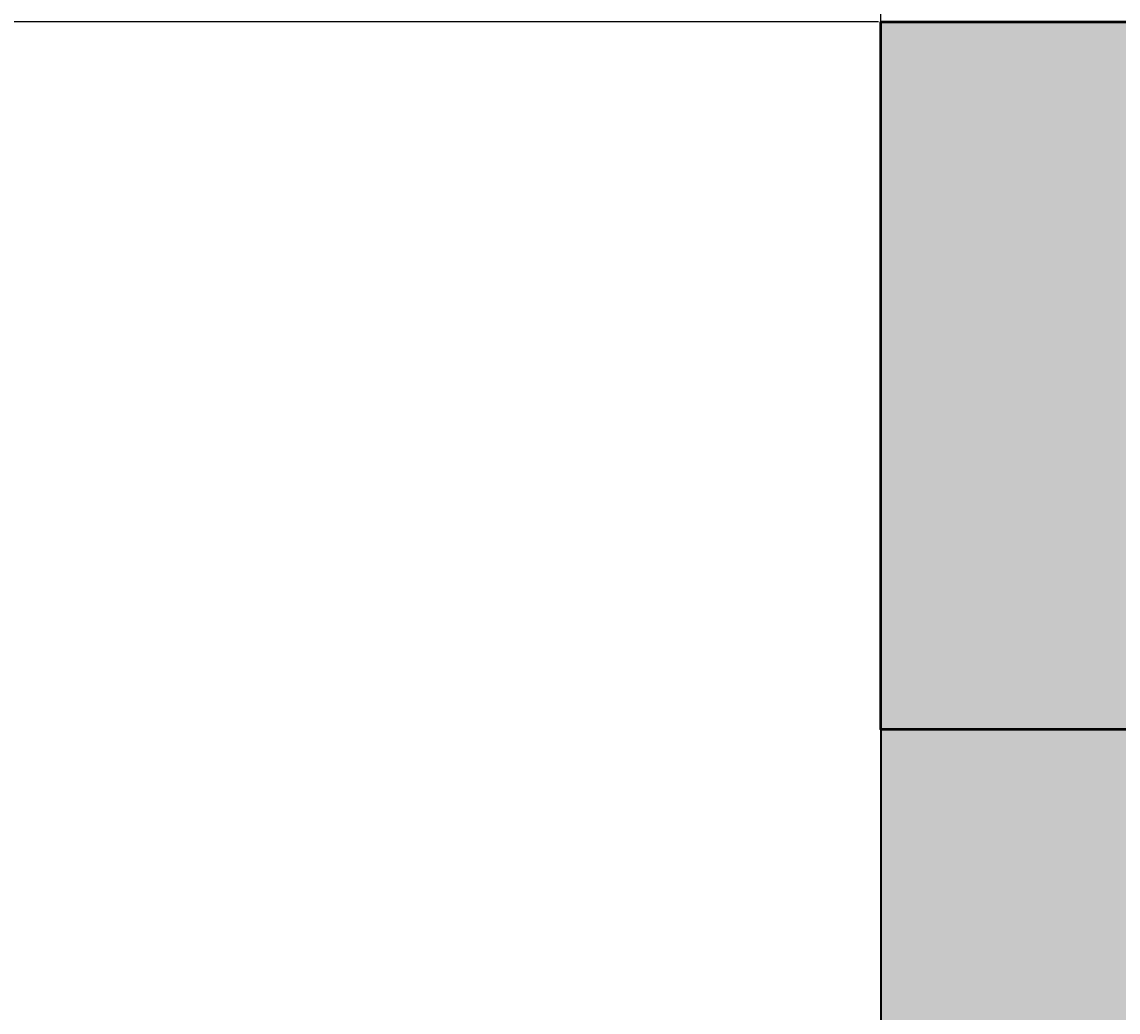
# Model space of a CAD drawing. Units: inches. Extents: x 1998 to 2588, y 1139 to 1977.
# Tile 71 of 134: x 2063 to 2095, y 1860 to 1889. Entities that reach past the tile are written whole.
import ezdxf

# ---------------------------------------------------------------- set-up
doc = ezdxf.new("R2010")
doc.units = ezdxf.units.IN
for name, color, linetype, lineweight in [('A-ANNO-DIMS', 2, 'Continuous', 18), ('A-COLS-PATT', 250, 'Continuous', 13), ('A-WALL-PATT', 252, 'Continuous', 13), ('COLUMN', 10, 'Continuous', 50), ('WALL', 200, 'Continuous', 35)]:
    doc.layers.add(name, color=color, linetype=linetype, lineweight=lineweight)
doc.styles.get("Standard").update_dxf_attribs({"font": 'arial.ttf'})
doc.dimstyles.get("Standard").update_dxf_attribs({"dimtxt": 0.18, "dimasz": 0.18, "dimexe": 0.18, "dimexo": 0.0625, "dimgap": 0.09, "dimtad": 0, "dimtih": 1, "dimtoh": 1, "dimdec": 4, "dimzin": 0, "dimdsep": 46, "dimtxsty": 'Standard', "dimcen": 0.09, "dimadec": 0, "dimazin": 0, "dimtfac": 1, "dimtdec": 4, "dimtofl": 0, "dimtmove": 0, "dimatfit": 3, "dimfxl": 1, "dimtolj": 1, "dimtzin": 0, "dimarcsym": 0})

# ---------------------------------------------------------------- blocks, each defined once
blk = doc.blocks.new('*D28')
at = {"layer": 'A-ANNO-DIMS', "color": 0, "lineweight": -2, "transparency": 16777216}
for p, q in [((2059.473, 1759.795), (2059.473, 1977.362)), ((2087.973, 1759.795), (2087.973, 1977.362)), ((2059.653, 1977.182), (2073.397, 1977.182)), ((2087.793, 1977.182), (2074.049, 1977.182))]:
    blk.add_line(p, q, dxfattribs=at)
at = {"layer": 'A-ANNO-DIMS', "color": 0, "transparency": 16777216}
for points in [[(2059.653, 1977.212), (2059.653, 1977.152), (2059.473, 1977.182)], [(2087.793, 1977.212), (2087.793, 1977.152), (2087.973, 1977.182)]]:
    blk.add_solid(points, dxfattribs=at)
at = {"layer": 'Defpoints', "color": 0, "transparency": 16777216}
for p in [(2087.973, 1977.182), (2059.473, 1759.732), (2087.973, 1759.732)]:
    blk.add_point(p, dxfattribs=at)
at = {"layer": 'A-ANNO-DIMS', "color": 0, "transparency": 16777216, "insert": (2073.723, 1977.182), "char_height": 0.18, "attachment_point": 5}
blk.add_mtext('\\A1;28.5', dxfattribs=at)
blk = doc.blocks.new('*D29')
at = {"layer": 'A-ANNO-DIMS', "color": 0, "lineweight": -2, "transparency": 16777216}
for p, q in [((2087.91, 1888.732), (1997.843, 1888.732)), ((1998.023, 1888.552), (1998.023, 1824.414)), ((1998.023, 1759.912), (1998.023, 1824.05)), ((2059.41, 1759.732), (1997.843, 1759.732))]:
    blk.add_line(p, q, dxfattribs=at)
at = {"layer": 'A-ANNO-DIMS', "color": 0, "transparency": 16777216}
for points in [[(1997.993, 1888.552), (1998.053, 1888.552), (1998.023, 1888.732)], [(1997.993, 1759.912), (1998.053, 1759.912), (1998.023, 1759.732)]]:
    blk.add_solid(points, dxfattribs=at)
at = {"layer": 'Defpoints', "color": 0, "transparency": 16777216}
for p in [(1998.023, 1888.732), (2087.973, 1888.732), (2059.473, 1759.732)]:
    blk.add_point(p, dxfattribs=at)
at = {"layer": 'A-ANNO-DIMS', "color": 0, "transparency": 16777216, "insert": (1998.023, 1824.232), "char_height": 0.18, "attachment_point": 5}
blk.add_mtext('\\A1;129', dxfattribs=at)

msp = doc.modelspace()

# ---------------------------------------------------------------- hatches: boundary and pattern name
at = {"layer": 'A-COLS-PATT'}
h = msp.add_hatch(color=256, dxfattribs=at)
h.dxf.hatch_style = 1
h.paths.add_polyline_path([(2099.4125, 1888.7324), (2087.9729, 1888.7324), (2087.9729, 1868.3278), (2099.4125, 1868.3278)])
h.paths.add_polyline_path([(2234.4125, 1888.7324), (2222.9729, 1888.7324), (2222.9729, 1868.3278), (2234.4125, 1868.3278)])
h.paths.add_polyline_path([(2341.4729, 1886.637), (2330.0332, 1886.637), (2330.0332, 1866.2324), (2341.4729, 1866.2324)])
h.paths.add_polyline_path([(2507.8006, 1882.7324), (2487.396, 1882.7324), (2487.396, 1871.2927), (2507.8006, 1871.2927)])
h.paths.add_polyline_path([(2510.9729, 1766.672), (2490.5682, 1766.672), (2490.5682, 1755.2324), (2510.9729, 1755.2324)])
h.paths.add_polyline_path([(2345.9729, 1759.7324), (2334.5332, 1759.7324), (2334.5332, 1739.3278), (2345.9729, 1739.3278)])
h.paths.add_polyline_path([(2234.4125, 1774.3318), (2222.9729, 1774.3318), (2222.9729, 1753.9272), (2234.4125, 1753.9272)])
h.paths.add_polyline_path([(2099.4125, 1775.637), (2087.9729, 1775.637), (2087.9729, 1755.2324), (2099.4125, 1755.2324)])
h.paths.add_polyline_path([(2098.0956, 1593.7241), (2077.691, 1593.7241), (2077.691, 1582.2845), (2098.0956, 1582.2845)])
h.paths.add_polyline_path([(2227.4729, 1604.637), (2216.0332, 1604.637), (2216.0332, 1584.2324), (2227.4729, 1584.2324)])
h.paths.add_polyline_path([(2345.9729, 1647.5211), (2334.5332, 1647.5211), (2334.5332, 1627.1165), (2345.9729, 1627.1165)])
h.paths.add_polyline_path([(2522.3775, 1641.2324), (2501.9729, 1641.2324), (2501.9729, 1629.7927), (2522.3775, 1629.7927)])
h.paths.add_polyline_path([(2522.3775, 1480.7324), (2501.9729, 1480.7324), (2501.9729, 1469.2927), (2522.3775, 1469.2927)])
h.paths.add_polyline_path([(2345.9729, 1488.5616), (2334.5332, 1488.5616), (2334.5332, 1468.1569), (2345.9729, 1468.1569)])
h.paths.add_polyline_path([(2234.4125, 1486.137), (2227.4729, 1486.137), (2227.4729, 1465.7324), (2234.4125, 1465.7324)])
h.paths.add_polyline_path([(2227.4729, 1486.137), (2222.9729, 1486.137), (2222.9729, 1465.7324), (2227.4729, 1465.7324)])
h.paths.add_polyline_path([(2108.3775, 1470.2324), (2087.9729, 1470.2324), (2087.9729, 1458.7927), (2108.3775, 1458.7927)])
h.paths.add_polyline_path([(2096.9729, 1365.5012), (2087.9729, 1365.5012), (2087.9729, 1345.0966), (2096.9729, 1345.0966)])
h.paths.add_polyline_path([(2087.9729, 1365.5012), (2085.5332, 1365.5012), (2085.5332, 1345.0966), (2087.9729, 1345.0966)])
h.paths.add_polyline_path([(2234.4125, 1285.137), (2222.9729, 1285.137), (2222.9729, 1264.7324), (2234.4125, 1264.7324)])
h.paths.add_polyline_path([(2345.9729, 1285.137), (2334.5332, 1285.137), (2334.5332, 1264.7324), (2345.9729, 1264.7324)])
h.paths.add_polyline_path([(2503.1458, 1240.172), (2482.7412, 1240.172), (2482.7412, 1228.7324), (2503.1458, 1228.7324)])
h.paths.add_polyline_path([(2510.9729, 1369.172), (2490.5682, 1369.172), (2490.5682, 1357.7324), (2510.9729, 1357.7324)])
at = {"layer": 'A-WALL-PATT'}
h = msp.add_hatch(color=256, dxfattribs=at)
h.dxf.hatch_style = 1
h.paths.add_polyline_path([(2222.9729, 1888.7324), (2099.4125, 1888.7324), (2099.4125, 1879.7324), (2222.9729, 1879.7324)])
h.paths.add_polyline_path([(2096.9729, 1868.3278), (2087.9729, 1868.3278), (2087.9729, 1775.637), (2096.9729, 1775.637)])
h.paths.add_polyline_path([(2227.4729, 1868.3278), (2222.9729, 1868.3278), (2222.9729, 1774.3318), (2227.4729, 1774.3318)])
h.paths.add_polyline_path([(2188.3019, 1759.7324), (2138.6074, 1759.7324), (2099.4125, 1759.7324), (2099.4125, 1755.2324), (2176.9729, 1755.2324), (2188.3019, 1755.2324)])
h.paths.add_polyline_path([(2087.9729, 1759.7324), (2059.4729, 1759.7324), (2059.4729, 1702.7324), (2087.9729, 1702.7324), (2087.9729, 1707.2324), (2063.9729, 1707.2324), (2063.9729, 1755.2324), (2087.9729, 1755.2324)])
h.paths.add_polyline_path([(2096.9729, 1755.2324), (2087.9729, 1755.2324), (2087.9729, 1707.2324), (2096.9729, 1707.2324)])
h.paths.add_polyline_path([(2187.0461, 1707.2324), (2105.9729, 1707.2324), (2096.9729, 1707.2324), (2087.9729, 1707.2324), (2087.9729, 1702.7324), (2105.9729, 1702.7324), (2114.9729, 1702.7324), (2187.0461, 1702.7324)])
h.paths.add_polyline_path([(2181.4729, 1719.2028), (2176.9729, 1719.2028), (2176.9729, 1707.2324), (2181.4729, 1707.2324)])
h.paths.add_polyline_path([(2216.0332, 1588.7324), (2114.9729, 1588.7324), (2105.9729, 1588.7324), (2105.9729, 1584.2324), (2216.0332, 1584.2324)])
h.paths.add_polyline_path([(2077.691, 1588.7324), (2061.4729, 1588.7324), (2061.4729, 1584.2324), (2077.691, 1584.2324)])
h.paths.add_polyline_path([(2105.9729, 1588.7324), (2098.0956, 1588.7324), (2098.0956, 1584.2324), (2105.9729, 1584.2324)])
h.paths.add_polyline_path([(2114.9729, 1596.2642), (2110.1012, 1596.2642), (2105.9729, 1596.2642), (2105.9729, 1588.7324), (2114.9729, 1588.7324)])
h.paths.add_polyline_path([(2114.9729, 1584.2324), (2105.9729, 1584.2324), (2105.9729, 1580.249), (2110.1012, 1580.249), (2114.9729, 1580.249)])
h.paths.add_polyline_path([(2114.9729, 1547.7716), (2110.1012, 1547.7716, -0.0318759), (2105.9729, 1548.035), (2105.9729, 1470.2324), (2108.3775, 1470.2324), (2108.3775, 1465.7324), (2186.2943, 1465.7324), (2186.2943, 1470.2324), (2114.9729, 1470.2324)])
h.paths.add_polyline_path([(2227.4729, 1584.2324), (2222.9729, 1584.2324), (2222.9729, 1486.137), (2227.4729, 1486.137)])
h.paths.add_polyline_path([(2295.4138, 1593.2324), (2227.4729, 1593.2324), (2227.4729, 1588.7324), (2295.4138, 1588.7324), (2295.4138, 1591.8729)])
h.paths.add_polyline_path([(2345.9729, 1627.1165), (2341.4729, 1627.1165), (2341.4729, 1593.2324), (2337.2869, 1593.2324), (2337.2869, 1591.8729), (2337.2869, 1588.7324), (2345.9729, 1588.7324)])
h.paths.add_polyline_path([(2291.9729, 1588.7324), (2287.4729, 1588.7324), (2287.4729, 1522.7324), (2291.9729, 1522.7324)])
h.paths.add_polyline_path([(2291.9729, 1522.7324), (2287.4729, 1522.7324), (2227.4729, 1522.7324), (2227.4729, 1518.2324), (2291.9729, 1518.2324)])
h.paths.add_polyline_path([(2295.7347, 1519.5919), (2295.7347, 1522.7324), (2291.9729, 1522.7324), (2291.9729, 1518.2324), (2295.7347, 1518.2324)])
h.paths.add_polyline_path([(2345.9729, 1522.7324), (2337.6078, 1522.7324), (2337.6078, 1519.5919), (2337.6078, 1518.2324), (2341.4729, 1518.2324), (2341.4729, 1488.5616), (2345.9729, 1488.5616)])
h.paths.add_polyline_path([(2345.9729, 1468.1569), (2341.4729, 1468.1569), (2341.4729, 1374.2324), (2227.4729, 1374.2324), (2227.4729, 1369.7324), (2345.9729, 1369.7324)])
h.paths.add_polyline_path([(2345.9729, 1369.7324), (2341.4729, 1369.7324), (2341.4729, 1362.2324), (2345.9729, 1362.2324)])
h.paths.add_polyline_path([(2345.9729, 1317.7324), (2345.9729, 1322.2324), (2341.4729, 1322.2324), (2341.4729, 1285.137), (2345.9729, 1285.137)], flags=17)
h.paths.add_polyline_path([(2356.2096, 1322.2324), (2345.9729, 1322.2324), (2345.9729, 1317.7324), (2356.2096, 1317.7324), (2356.2096, 1319.3088)], flags=17)
h.paths.add_polyline_path([(2393.9729, 1322.2324), (2375.6999, 1322.2324), (2375.6999, 1319.3088, -0.0202458), (2375.636, 1317.7324), (2393.9729, 1317.7324)], flags=17)
h.paths.add_polyline_path([(2398.4729, 1322.2324), (2393.9729, 1322.2324), (2393.9729, 1317.7324), (2393.9729, 1237.7324), (2345.9729, 1237.7324), (2345.9729, 1264.7324), (2341.4729, 1264.7324), (2341.4729, 1228.7324), (2393.9729, 1228.7324), (2482.7412, 1228.7324), (2482.7412, 1237.7324), (2398.4729, 1237.7324), (2398.4729, 1297.1029)])
h.paths.add_polyline_path([(2398.4729, 1362.2324), (2393.9729, 1362.2324), (2393.9729, 1357.7324), (2398.4729, 1357.7324)])
h.paths.add_polyline_path([(2345.9729, 1329.7549), (2341.4729, 1329.7549), (2341.4729, 1322.2324), (2345.9729, 1322.2324)])

# ---------------------------------------------------------------- linework, layer by layer
at = {"layer": 'COLUMN'}
msp.add_lwpolyline([(2087.9729, 1888.7324), (2099.4125, 1888.7324), (2099.4125, 1868.3278), (2087.9729, 1868.3278)], close=True, dxfattribs=at)
at = {"layer": 'WALL'}
for p, q in [((2227.4729, 1888.7324), (2087.9729, 1888.7324)), ((2087.9729, 1888.7324), (2087.9729, 1755.2324))]:
    msp.add_line(p, q, dxfattribs=at)

# ---------------------------------------------------------------- dimensions: what is measured, and where the dimension line sits
at = {"layer": 'A-ANNO-DIMS'}
dim = msp.add_linear_dim(base=(2087.9729, 1977.1824), p1=(2059.4729, 1759.7324), p2=(2087.9729, 1759.7324), dimstyle='Standard', override={"dimdec": 1, "dimlfac": 1, "dimrnd": 0, "dimzin": 0, "dimdsep": 46, "dimlunit": 2}, dxfattribs=at)
dim.commit()
dim.dimension.update_dxf_attribs({"geometry": '*D28', "text_midpoint": (2073.7229, 1977.1824)})
dim = msp.add_linear_dim(base=(1998.0229, 1888.7324), p1=(2059.4729, 1759.7324), p2=(2087.9729, 1888.7324), angle=90, dimstyle='Standard', override={"dimdec": 0, "dimlfac": 1, "dimrnd": 0, "dimzin": 0, "dimdsep": 46, "dimlunit": 2}, dxfattribs=at)
dim.commit()
dim.dimension.update_dxf_attribs({"geometry": '*D29', "text_midpoint": (1998.0229, 1824.2324)})

doc.saveas('drawing.dxf')
